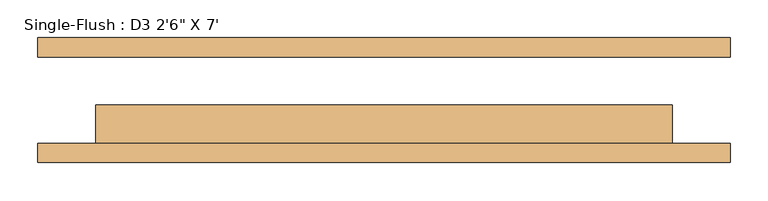
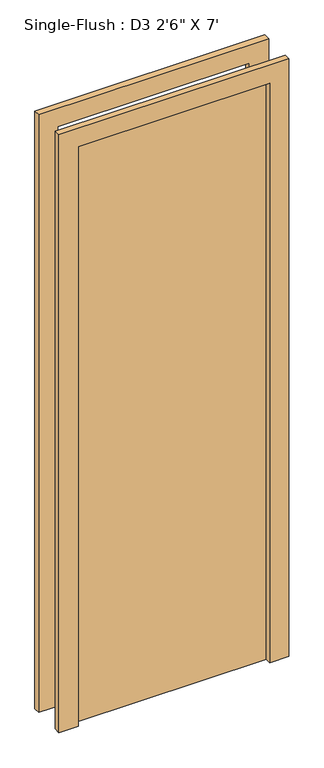
"""IFC4 building model written with IfcOpenShell, lengths in millimetres: door geometry."""

from ifc_helpers import new_model, si_unit, frame, origin, origin_with_axes, place, context, project, spatial, polyline, outline, extrude, source, transform, mapped, element, save


def door_019bc352(model_context):
    return source(origin(), model_context, "Body", "SweptSolid", [
        extrude(outline(polyline([(2514.6, -457.2), (0.0, -457.2), (0.0, -381.0), (2438.4, -381.0), (2438.4, 381.0), (0.0, 381.0), (0.0, 457.2), (2514.6, 457.2), (2514.6, -457.2)])), frame((0.0, -82.55, 0.0), z_axis=(0.0, 1.0, 0.0), x_axis=(0.0, 0.0, 1.0)), (0.0, 0.0, 1.0), 25.4),
        extrude(outline(polyline([(2514.6, 457.2), (2514.6, -457.2), (0.0, -457.2), (0.0, -381.0), (2438.4, -381.0), (2438.4, 381.0), (0.0, 381.0), (0.0, 457.2), (2514.6, 457.2)])), frame((0.0, 57.15, 0.0), z_axis=(0.0, 1.0, 0.0), x_axis=(0.0, 0.0, 1.0)), (0.0, 0.0, 1.0), 25.4),
        extrude(outline(polyline([(381.0, -6.35), (381.0, -57.15), (-381.0, -57.15), (-381.0, -6.35), (381.0, -6.35)])), origin_with_axes(), (0.0, 0.0, 1.0), 2438.4),
    ])


if __name__ == "__main__":
    model = new_model("IFC4")
    model_context = context("Model", 3, world=origin())
    ifc_project = project(units=[si_unit("LENGTHUNIT", "METRE", prefix="MILLI")], contexts=[model_context])
    site = spatial("IfcSite", under=ifc_project)
    building = spatial("IfcBuilding", under=site)
    placement = place(None, origin())
    door_shape = door_019bc352(model_context)
    element("IfcDoor", 1, ObjectType="Single-Flush : D3 2'6\" X 7'", at=placement, inside=building, context=model_context, shape_type="MappedRepresentation", body=[
        mapped(door_shape, transform((0.0, 0.0, 0.0), x_axis=(1.0, 0.0, 0.0), y_axis=(0.0, 1.0, 0.0), z_axis=(0.0, 0.0, 1.0))),
    ])
    save(model, "model.ifc")

# Revit data of these elements
# Type "Single-Flush : D3 2'6\" X 7'"
#   Type Mark = "11"
#   Construction Type Id = "MDOOR"
#   Assembly Code = "C1020"
#   Analytic Construction = "Metal"
#   Thickness = 0' - 2"
#   Heat Transfer Coefficient (U) = 0.651978 BTU/(h·ft²·°F)
#   Height = 8' - 0"
#   Trim Projection Ext = 0' - 1"
#   Trim Projection Int = 0' - 1"
#   Trim Width = 0' - 3"
#   Width = 2' - 6"
#   Define Thermal Properties by = 1
#   Door Material = Door - Panel
#   Frame Material = Door - Frame
#   Visual Light Transmittance = 0
#   Solar Heat Gain Coefficient = 0
#   Function = (empty or 0)
#   Wall Closure = (empty or 0)
# Element 1 (IfcDoor, "Single-Flush : D3 2'6\" X 7'")
#   Materials on its faces: "Door - Frame", "Door - Panel"
# Materials
#   "Door - Panel": class "Wood", colour RGB 210 159 95, transparency 0, Cost = 0
#   "Door - Frame": colour RGB 118 70 51, transparency 0, Cost = 0
